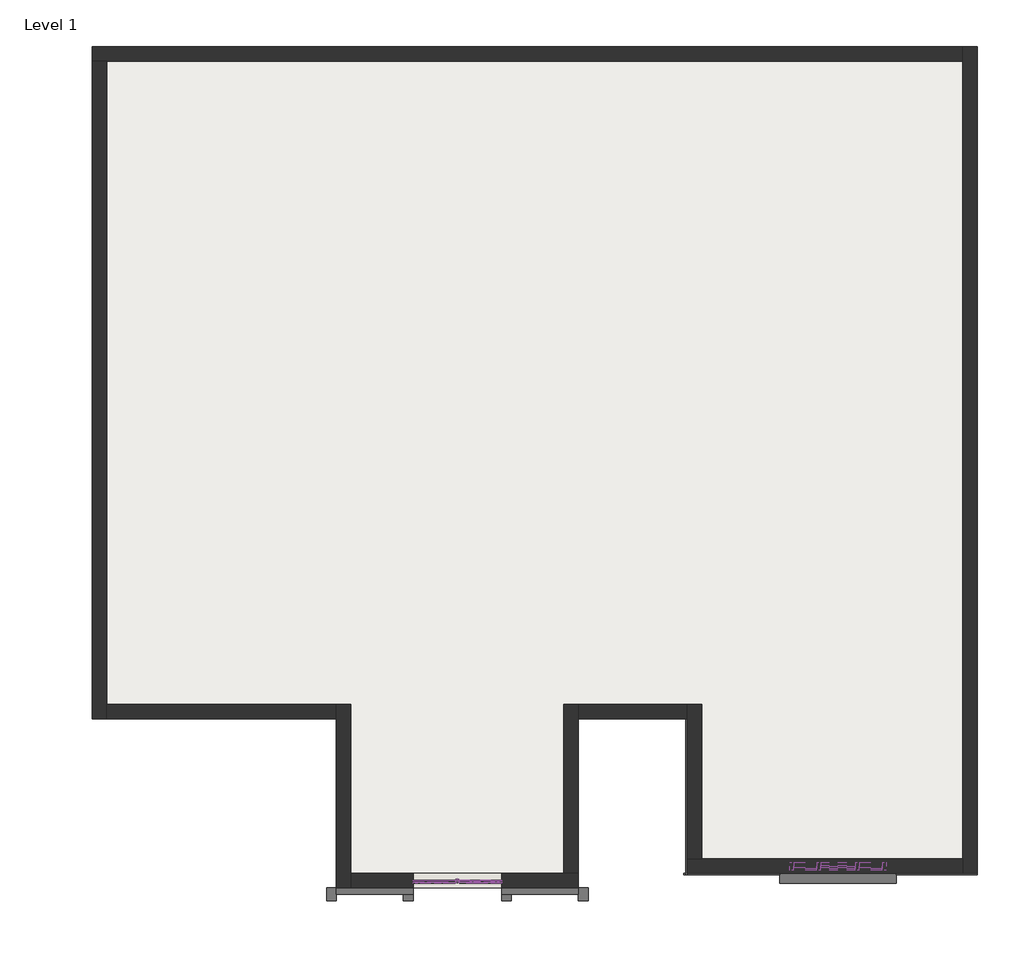
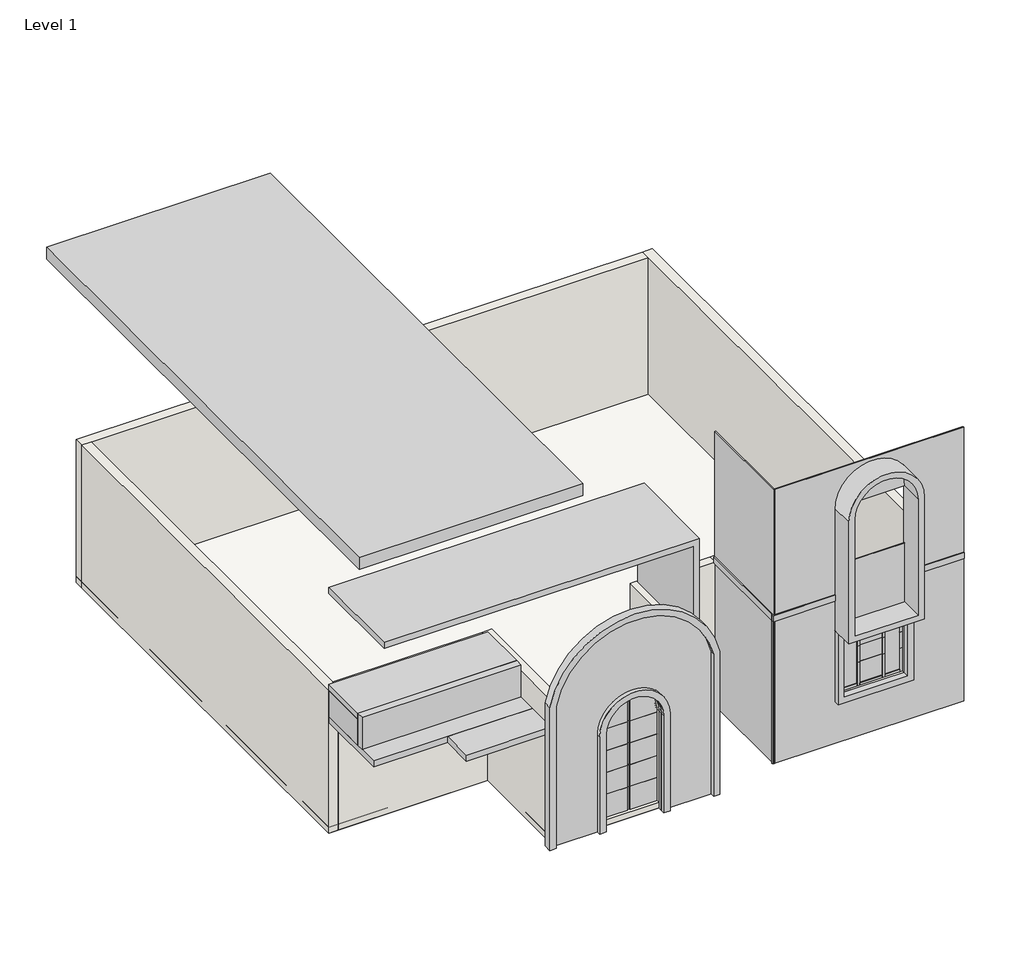
# One storey: 52 members, 17 plates, 10 walls, 1 proxy, 1 slab.
"""IFC4 building model written with IfcOpenShell, lengths in millimetres."""

from ifc_helpers import new_model, si_unit, frame, origin, origin_with_axes, place, context, project, spatial, polyline, circle_curve, outline, extrude, faceted_brep, transform, mapped, element, save
from ifc_brep_helpers import plane_surface, revolved_surface, advanced_brep
from components import generic_models_1_generic_models_1_ec26760c, member_08c7225e, member_28930b13, member_e49bab3c, member_1c8f807b, member_b3cb6624, member_4e015be9, member_3b441234, member_02ee8d56, member_e1a7572e, member_43115751, member_bd529d22, member_a55882dd, member_6e035839, member_ea2f4e14, member_6b6d42fb, member_11e54509, member_471b44ca, member_90750a43, member_576e3203, member_843225dc, member_a980948f, member_7fd687a9, member_94122dd8, member_cc20b924, system_panel_glazed_54165e4b, system_panel_glazed_81b96659, system_panel_glazed_ec3758d8, system_panel_glazed_692768b6, system_panel_glazed_4eb050cd, system_panel_glazed_dbe48e5a, system_panel_glazed_09ca6336, system_panel_glazed_22d47ebb, system_panel_glazed_ec18a58b, system_panel_glazed_47dd2052

model = new_model("IFC4")

# Units and contexts
model_context = context("Model", 3, world=origin())
ifc_project = project(units=[si_unit("LENGTHUNIT", "METRE", prefix="MILLI")], contexts=[model_context])

# Site, building, storey
site = spatial("IfcSite", under=ifc_project)
building = spatial("IfcBuilding", under=site)
storey = spatial("IfcBuildingStorey", under=building, Name="Level 1", Elevation=0.0)

# Proxy
placement = place(None, origin())
generic_models_1_generic_models_1_shape = generic_models_1_generic_models_1_ec26760c(model_context)
element("IfcBuildingElementProxy", 1, Name="Generic Models 1 : Generic Models 1", ObjectType="Generic Models 1 : Generic Models 1", at=placement, inside=storey, context=model_context, shape_type="MappedRepresentation", body=[
    mapped(generic_models_1_generic_models_1_shape, transform((0.0, 0.0, 0.0), x_axis=(1.0, 0.0, 0.0), y_axis=(0.0, 1.0, 0.0), z_axis=(0.0, 0.0, 1.0))),
])

# Members
member_shape = member_08c7225e(model_context)
element("IfcMember", 2, ObjectType="Circular Mullion : 2.5\" Circular", at=placement, inside=storey, context=model_context, shape_type="MappedRepresentation", body=[
    mapped(member_shape, transform((-633.8864268, -1847.4234736, 745.0666667), x_axis=(-1.0, 0.0, 0.0), y_axis=(0.0, 1.0, 0.0), z_axis=(0.0, 0.0, -1.0))),
])
element("IfcMember", 3, ObjectType="Circular Mullion : 2.5\" Circular", at=placement, inside=storey, context=model_context, shape_type="MappedRepresentation", body=[
    mapped(member_shape, transform((-633.8864268, -1847.4234736, 1303.8666667), x_axis=(-1.0, 0.0, 0.0), y_axis=(0.0, 1.0, 0.0), z_axis=(0.0, 0.0, -1.0))),
])
element("IfcMember", 4, ObjectType="Circular Mullion : 2.5\" Circular", at=placement, inside=storey, context=model_context, shape_type="MappedRepresentation", body=[
    mapped(member_shape, transform((-633.8864268, -1847.4234736, 1862.6666667), x_axis=(-1.0, 0.0, 0.0), y_axis=(0.0, 1.0, 0.0), z_axis=(0.0, 0.0, -1.0))),
])
member_2_shape = member_28930b13(model_context)
element("IfcMember", 5, ObjectType="Circular Mullion : 2.5\" Circular", at=placement, inside=storey, context=model_context, shape_type="MappedRepresentation", body=[
    mapped(member_2_shape, transform((-633.8864268, -1847.4234736, 2421.4666667), x_axis=(-1.0, 0.0, 0.0), y_axis=(0.0, 1.0, 0.0), z_axis=(0.0, 0.0, -1.0))),
])
member_3_shape = member_e49bab3c(model_context)
element("IfcMember", 6, ObjectType="Circular Mullion : 2.5\" Circular", at=placement, inside=storey, context=model_context, shape_type="MappedRepresentation", body=[
    mapped(member_3_shape, transform((-633.8864268, -1847.4234736, 3048.0), x_axis=(-1.0, 0.0, 0.0), y_axis=(0.0, 1.0, 0.0), z_axis=(0.0, 0.0, -1.0))),
])
member_4_shape = member_1c8f807b(model_context)
element("IfcMember", 7, ObjectType="Circular Mullion : 2.5\" Circular", at=placement, inside=storey, context=model_context, shape_type="MappedRepresentation", body=[
    mapped(member_4_shape, transform((-633.8864268, -1847.4234736, 152.4), x_axis=(-1.0, 0.0, 0.0), y_axis=(0.0, 1.0, 0.0), z_axis=(0.0, 0.0, -1.0))),
])
member_5_shape = member_b3cb6624(model_context)
element("IfcMember", 8, ObjectType="Circular Mullion : 2.5\" Circular 2", at=placement, inside=storey, context=model_context, shape_type="MappedRepresentation", body=[
    mapped(member_5_shape, transform((-1052.9864268, -1847.4234736, 3048.0), x_axis=(0.0, 0.0, 1.0), y_axis=(0.0, 1.0, 0.0), z_axis=(-1.0, 0.0, 0.0))),
])
element("IfcMember", 9, ObjectType="Circular Mullion : 2.5\" Circular 2", at=placement, inside=storey, context=model_context, shape_type="MappedRepresentation", body=[
    mapped(member_5_shape, transform((-602.1364268, -1847.4234736, 3048.0), x_axis=(0.0, 0.0, 1.0), y_axis=(0.0, 1.0, 0.0), z_axis=(-1.0, 0.0, 0.0))),
])
member_6_shape = member_4e015be9(model_context)
element("IfcMember", 10, ObjectType="Circular Mullion : 2.5\" Circular 2", at=placement, inside=storey, context=model_context, shape_type="MappedRepresentation", body=[
    mapped(member_6_shape, transform((-1325.1474268, -1847.4234736, 1862.6666667), x_axis=(0.0, 0.0, 1.0), y_axis=(0.0, 1.0, 0.0), z_axis=(-1.0, 0.0, 0.0))),
])
element("IfcMember", 11, ObjectType="Circular Mullion : 2.5\" Circular 2", at=placement, inside=storey, context=model_context, shape_type="MappedRepresentation", body=[
    mapped(member_6_shape, transform((-602.1364268, -1847.4234736, 1862.6666667), x_axis=(0.0, 0.0, 1.0), y_axis=(0.0, 1.0, 0.0), z_axis=(-1.0, 0.0, 0.0))),
])
element("IfcMember", 12, ObjectType="Circular Mullion : 2.5\" Circular 2", at=placement, inside=storey, context=model_context, shape_type="MappedRepresentation", body=[
    mapped(member_6_shape, transform((-1325.1474268, -1847.4234736, 1303.8666667), x_axis=(0.0, 0.0, 1.0), y_axis=(0.0, 1.0, 0.0), z_axis=(-1.0, 0.0, 0.0))),
])
element("IfcMember", 13, ObjectType="Circular Mullion : 2.5\" Circular 2", at=placement, inside=storey, context=model_context, shape_type="MappedRepresentation", body=[
    mapped(member_6_shape, transform((-602.1364268, -1847.4234736, 1303.8666667), x_axis=(0.0, 0.0, 1.0), y_axis=(0.0, 1.0, 0.0), z_axis=(-1.0, 0.0, 0.0))),
])
element("IfcMember", 14, ObjectType="Circular Mullion : 2.5\" Circular 2", at=placement, inside=storey, context=model_context, shape_type="MappedRepresentation", body=[
    mapped(member_6_shape, transform((-1325.1474268, -1847.4234736, 745.0666667), x_axis=(0.0, 0.0, 1.0), y_axis=(0.0, 1.0, 0.0), z_axis=(-1.0, 0.0, 0.0))),
])
element("IfcMember", 15, ObjectType="Circular Mullion : 2.5\" Circular 2", at=placement, inside=storey, context=model_context, shape_type="MappedRepresentation", body=[
    mapped(member_6_shape, transform((-602.1364268, -1847.4234736, 745.0666667), x_axis=(0.0, 0.0, 1.0), y_axis=(0.0, 1.0, 0.0), z_axis=(-1.0, 0.0, 0.0))),
])
element("IfcMember", 16, ObjectType="Circular Mullion : 2.5\" Circular 2", at=placement, inside=storey, context=model_context, shape_type="MappedRepresentation", body=[
    mapped(member_6_shape, transform((-1325.1474268, -1847.4234736, 2421.4666667), x_axis=(0.0, 0.0, 1.0), y_axis=(0.0, 1.0, 0.0), z_axis=(-1.0, 0.0, 0.0))),
])
member_7_shape = member_3b441234(model_context)
element("IfcMember", 17, ObjectType="Circular Mullion : 2.5\" Circular 2", at=placement, inside=storey, context=model_context, shape_type="MappedRepresentation", body=[
    mapped(member_7_shape, transform((64.6135732, -1847.4234736, 2489.2), x_axis=(1.0, 0.0, 0.0), y_axis=(0.0, 1.0, 0.0), z_axis=(0.0, 0.0, 1.0))),
])
member_8_shape = member_02ee8d56(model_context)
element("IfcMember", 18, ObjectType="Circular Mullion : 2.5\" Circular 2", at=placement, inside=storey, context=model_context, shape_type="MappedRepresentation", body=[
    mapped(member_8_shape, transform((-1332.3864268, -1847.4234736, 152.4), x_axis=(-1.0, 0.0, 0.0), y_axis=(0.0, 1.0, 0.0), z_axis=(0.0, 0.0, -1.0))),
])
member_9_shape = member_e1a7572e(model_context)
element("IfcMember", 19, ObjectType="Circular Mullion : 2.5\" Circular 2", at=placement, inside=storey, context=model_context, shape_type="MappedRepresentation", body=[
    mapped(member_9_shape, transform((57.3745732, -1847.4234736, 152.4), x_axis=(0.0, 0.0, -1.0), y_axis=(0.0, 1.0, 0.0), z_axis=(1.0, 0.0, 0.0))),
])
element("IfcMember", 20, ObjectType="Circular Mullion : 2.5\" Circular 2", at=placement, inside=storey, context=model_context, shape_type="MappedRepresentation", body=[
    mapped(member_9_shape, transform((-665.6364268, -1847.4234736, 152.4), x_axis=(0.0, 0.0, -1.0), y_axis=(0.0, 1.0, 0.0), z_axis=(1.0, 0.0, 0.0))),
])
member_10_shape = member_43115751(model_context)
element("IfcMember", 21, ObjectType="Circular Mullion : 2.5\" Circular 2", at=placement, inside=storey, context=model_context, shape_type="MappedRepresentation", body=[
    mapped(member_10_shape, transform((-1332.3864268, -1847.4234736, 2489.2), x_axis=(-1.0, 0.0, 0.0), y_axis=(0.0, 1.0, 0.0), z_axis=(0.0, 0.0, -1.0))),
])
element("IfcMember", 22, ObjectType="Circular Mullion : 2.5\" Circular 2", at=placement, inside=storey, context=model_context, shape_type="MappedRepresentation", body=[
    mapped(member_7_shape, transform((-1332.3864268, -1847.4234736, 2421.4666667), x_axis=(-1.0, 0.0, 0.0), y_axis=(0.0, 1.0, 0.0), z_axis=(0.0, 0.0, -1.0))),
])
member_11_shape = member_bd529d22(model_context)
element("IfcMember", 23, ObjectType="Circular Mullion : 2.5\" Circular 2", at=placement, inside=storey, context=model_context, shape_type="MappedRepresentation", body=[
    mapped(member_11_shape, transform((-1332.3864268, -1847.4234736, 1862.6666667), x_axis=(-1.0, 0.0, 0.0), y_axis=(0.0, 1.0, 0.0), z_axis=(0.0, 0.0, -1.0))),
])
element("IfcMember", 24, ObjectType="Circular Mullion : 2.5\" Circular 2", at=placement, inside=storey, context=model_context, shape_type="MappedRepresentation", body=[
    mapped(member_11_shape, transform((-1332.3864268, -1847.4234736, 1303.8666667), x_axis=(-1.0, 0.0, 0.0), y_axis=(0.0, 1.0, 0.0), z_axis=(0.0, 0.0, -1.0))),
])
element("IfcMember", 25, ObjectType="Circular Mullion : 2.5\" Circular 2", at=placement, inside=storey, context=model_context, shape_type="MappedRepresentation", body=[
    mapped(member_11_shape, transform((-1332.3864268, -1847.4234736, 745.0666667), x_axis=(-1.0, 0.0, 0.0), y_axis=(0.0, 1.0, 0.0), z_axis=(0.0, 0.0, -1.0))),
])
element("IfcMember", 26, ObjectType="Circular Mullion : 2.5\" Circular 2", at=placement, inside=storey, context=model_context, shape_type="MappedRepresentation", body=[
    mapped(member_11_shape, transform((64.6135732, -1847.4234736, 2421.4666667), x_axis=(1.0, 0.0, 0.0), y_axis=(0.0, 1.0, 0.0), z_axis=(0.0, 0.0, 1.0))),
])
element("IfcMember", 27, ObjectType="Circular Mullion : 2.5\" Circular 2", at=placement, inside=storey, context=model_context, shape_type="MappedRepresentation", body=[
    mapped(member_11_shape, transform((64.6135732, -1847.4234736, 1862.6666667), x_axis=(1.0, 0.0, 0.0), y_axis=(0.0, 1.0, 0.0), z_axis=(0.0, 0.0, 1.0))),
])
element("IfcMember", 28, ObjectType="Circular Mullion : 2.5\" Circular 2", at=placement, inside=storey, context=model_context, shape_type="MappedRepresentation", body=[
    mapped(member_11_shape, transform((64.6135732, -1847.4234736, 1303.8666667), x_axis=(1.0, 0.0, 0.0), y_axis=(0.0, 1.0, 0.0), z_axis=(0.0, 0.0, 1.0))),
])
element("IfcMember", 29, ObjectType="Circular Mullion : 2.5\" Circular 2", at=placement, inside=storey, context=model_context, shape_type="MappedRepresentation", body=[
    mapped(member_8_shape, transform((64.6135732, -1847.4234736, 745.0666667), x_axis=(1.0, 0.0, 0.0), y_axis=(0.0, 1.0, 0.0), z_axis=(0.0, 0.0, 1.0))),
])
member_12_shape = member_a55882dd(model_context)
element("IfcMember", 30, ObjectType="Circular Mullion : 2.5\" Circular 2", at=placement, inside=storey, context=model_context, shape_type="MappedRepresentation", body=[
    mapped(member_12_shape, transform((-633.8864268, -1847.4234736, 3187.7), x_axis=(0.0, 0.0, 1.0), y_axis=(0.0, 1.0, 0.0), z_axis=(-1.0, 0.0, 0.0))),
])
member_13_shape = member_6e035839(model_context)
element("IfcMember", 31, ObjectType="Circular Mullion : 2.5\" Circular 2", at=placement, inside=storey, context=model_context, shape_type="MappedRepresentation", body=[
    mapped(member_13_shape, transform((-214.7864268, -1847.4234736, 3048.0), x_axis=(0.5999999999999911, 0.0, 0.8000000000000067), y_axis=(0.0, 1.0, 0.0), z_axis=(-0.8000000000000067, 0.0, 0.5999999999999911))),
])
member_14_shape = member_ea2f4e14(model_context)
element("IfcMember", 32, ObjectType="Circular Mullion : 2.5\" Circular 2", at=placement, inside=storey, context=model_context, shape_type="MappedRepresentation", body=[
    mapped(member_14_shape, transform((-1052.9864268, -1847.4234736, 3048.0), x_axis=(-0.5999999999999878, 0.0, 0.8000000000000093), y_axis=(0.0, 1.0, 0.0), z_axis=(-0.8000000000000091, 0.0, -0.5999999999999877))),
])
member_15_shape = member_6b6d42fb(model_context)
element("IfcMember", 33, ObjectType="Rectangular Mullion : 1\" Square", at=placement, inside=storey, context=model_context, shape_type="MappedRepresentation", body=[
    mapped(member_15_shape, transform((-602.1364268, -1847.4234736, 2421.4666667), x_axis=(0.0, 0.0, 1.0), y_axis=(0.0, 1.0, 0.0), z_axis=(-1.0, 0.0, 0.0))),
])
member_16_shape = member_11e54509(model_context)
element("IfcMember", 34, ObjectType="Rectangular Mullion : 1\" Square", at=placement, inside=storey, context=model_context, shape_type="MappedRepresentation", body=[
    mapped(member_16_shape, transform((5087.4635732, -1618.8234736, 2235.2), x_axis=(0.0, 0.0, 1.0), y_axis=(0.0, 1.0, 0.0), z_axis=(-1.0, 0.0, 0.0))),
])
element("IfcMember", 35, ObjectType="Rectangular Mullion : 1\" Square", at=placement, inside=storey, context=model_context, shape_type="MappedRepresentation", body=[
    mapped(member_16_shape, transform((5087.4635732, -1618.8234736, 1820.3333333), x_axis=(0.0, 0.0, 1.0), y_axis=(0.0, 1.0, 0.0), z_axis=(-1.0, 0.0, 0.0))),
])
member_17_shape = member_471b44ca(model_context)
element("IfcMember", 36, ObjectType="Rectangular Mullion : 2.5\" x 5\" rectangular", at=placement, inside=storey, context=model_context, shape_type="MappedRepresentation", body=[
    mapped(member_17_shape, transform((5055.7135732, -1618.8234736, 1820.3333333), x_axis=(-1.0, 0.0, 0.0), y_axis=(0.0, 1.0, 0.0), z_axis=(0.0, 0.0, -1.0))),
])
element("IfcMember", 37, ObjectType="Rectangular Mullion : 2.5\" x 5\" rectangular", at=placement, inside=storey, context=model_context, shape_type="MappedRepresentation", body=[
    mapped(member_17_shape, transform((5665.3135732, -1618.8234736, 1820.3333333), x_axis=(-1.0, 0.0, 0.0), y_axis=(0.0, 1.0, 0.0), z_axis=(0.0, 0.0, -1.0))),
])
member_18_shape = member_90750a43(model_context)
element("IfcMember", 38, ObjectType="Rectangular Mullion : 2.5\" x 5\" rectangular", at=placement, inside=storey, context=model_context, shape_type="MappedRepresentation", body=[
    mapped(member_18_shape, transform((5055.7135732, -1618.8234736, 2235.2), x_axis=(-1.0, 0.0, 0.0), y_axis=(0.0, 1.0, 0.0), z_axis=(0.0, 0.0, -1.0))),
])
element("IfcMember", 39, ObjectType="Rectangular Mullion : 2.5\" x 5\" rectangular", at=placement, inside=storey, context=model_context, shape_type="MappedRepresentation", body=[
    mapped(member_18_shape, transform((5665.3135732, -1618.8234736, 2235.2), x_axis=(-1.0, 0.0, 0.0), y_axis=(0.0, 1.0, 0.0), z_axis=(0.0, 0.0, -1.0))),
])
member_19_shape = member_576e3203(model_context)
element("IfcMember", 40, ObjectType="Rectangular Mullion : 2.5\" x 5\" rectangular", at=placement, inside=storey, context=model_context, shape_type="MappedRepresentation", body=[
    mapped(member_19_shape, transform((5055.7135732, -1618.8234736, 1219.2), x_axis=(-1.0, 0.0, 0.0), y_axis=(0.0, 1.0, 0.0), z_axis=(0.0, 0.0, -1.0))),
])
element("IfcMember", 41, ObjectType="Rectangular Mullion : 2.5\" x 5\" rectangular", at=placement, inside=storey, context=model_context, shape_type="MappedRepresentation", body=[
    mapped(member_19_shape, transform((5665.3135732, -1618.8234736, 1219.2), x_axis=(-1.0, 0.0, 0.0), y_axis=(0.0, 1.0, 0.0), z_axis=(0.0, 0.0, -1.0))),
])
member_20_shape = member_843225dc(model_context)
element("IfcMember", 42, ObjectType="Rectangular Mullion : 2.5\" x 5\" rectangular", at=placement, inside=storey, context=model_context, shape_type="MappedRepresentation", body=[
    mapped(member_20_shape, transform((4662.0135732, -1618.8234736, 2743.2), x_axis=(0.0, 0.0, 1.0), y_axis=(0.0, 1.0, 0.0), z_axis=(-1.0, 0.0, 0.0))),
])
element("IfcMember", 43, ObjectType="Rectangular Mullion : 2.5\" x 5\" rectangular", at=placement, inside=storey, context=model_context, shape_type="MappedRepresentation", body=[
    mapped(member_20_shape, transform((5697.0635732, -1618.8234736, 2743.2), x_axis=(0.0, 0.0, 1.0), y_axis=(0.0, 1.0, 0.0), z_axis=(-1.0, 0.0, 0.0))),
])
element("IfcMember", 44, ObjectType="Rectangular Mullion : 2.5\" x 5\" rectangular", at=placement, inside=storey, context=model_context, shape_type="MappedRepresentation", body=[
    mapped(member_20_shape, transform((6059.0135732, -1618.8234736, 1219.2), x_axis=(0.0, 0.0, -1.0), y_axis=(0.0, 1.0, 0.0), z_axis=(1.0, 0.0, 0.0))),
])
element("IfcMember", 45, ObjectType="Rectangular Mullion : 2.5\" x 5\" rectangular", at=placement, inside=storey, context=model_context, shape_type="MappedRepresentation", body=[
    mapped(member_20_shape, transform((5023.9635732, -1618.8234736, 1219.2), x_axis=(0.0, 0.0, -1.0), y_axis=(0.0, 1.0, 0.0), z_axis=(1.0, 0.0, 0.0))),
])
member_21_shape = member_a980948f(model_context)
element("IfcMember", 46, ObjectType="Rectangular Mullion : 2.5\" x 5\" rectangular", at=placement, inside=storey, context=model_context, shape_type="MappedRepresentation", body=[
    mapped(member_21_shape, transform((5633.5635732, -1618.8234736, 1219.2), x_axis=(0.0, 0.0, -1.0), y_axis=(0.0, 1.0, 0.0), z_axis=(1.0, 0.0, 0.0))),
])
element("IfcMember", 47, ObjectType="Rectangular Mullion : 2.5\" x 5\" rectangular", at=placement, inside=storey, context=model_context, shape_type="MappedRepresentation", body=[
    mapped(member_21_shape, transform((5087.4635732, -1618.8234736, 2743.2), x_axis=(0.0, 0.0, 1.0), y_axis=(0.0, 1.0, 0.0), z_axis=(-1.0, 0.0, 0.0))),
])
member_22_shape = member_7fd687a9(model_context)
element("IfcMember", 48, ObjectType="Rectangular Mullion : 2.5\" x 5\" rectangular", at=placement, inside=storey, context=model_context, shape_type="MappedRepresentation", body=[
    mapped(member_22_shape, transform((6122.5135732, -1618.8234736, 2743.2), x_axis=(1.0, 0.0, 0.0), y_axis=(0.0, 1.0, 0.0), z_axis=(0.0, 0.0, 1.0))),
])
member_23_shape = member_94122dd8(model_context)
element("IfcMember", 49, ObjectType="Rectangular Mullion : 2.5\" x 5\" rectangular", at=placement, inside=storey, context=model_context, shape_type="MappedRepresentation", body=[
    mapped(member_23_shape, transform((4598.5135732, -1618.8234736, 1219.2), x_axis=(-1.0, 0.0, 0.0), y_axis=(0.0, 1.0, 0.0), z_axis=(0.0, 0.0, -1.0))),
])
element("IfcMember", 50, ObjectType="Rectangular Mullion : 2.5\" x 5\" rectangular", at=placement, inside=storey, context=model_context, shape_type="MappedRepresentation", body=[
    mapped(member_22_shape, transform((4598.5135732, -1618.8234736, 2235.2), x_axis=(-1.0, 0.0, 0.0), y_axis=(0.0, 1.0, 0.0), z_axis=(0.0, 0.0, -1.0))),
])
member_24_shape = member_cc20b924(model_context)
element("IfcMember", 51, ObjectType="Rectangular Mullion : 2.5\" x 5\" rectangular", at=placement, inside=storey, context=model_context, shape_type="MappedRepresentation", body=[
    mapped(member_24_shape, transform((4598.5135732, -1618.8234736, 1820.3333333), x_axis=(-1.0, 0.0, 0.0), y_axis=(0.0, 1.0, 0.0), z_axis=(0.0, 0.0, -1.0))),
])
element("IfcMember", 52, ObjectType="Rectangular Mullion : 2.5\" x 5\" rectangular", at=placement, inside=storey, context=model_context, shape_type="MappedRepresentation", body=[
    mapped(member_24_shape, transform((6122.5135732, -1618.8234736, 2235.2), x_axis=(1.0, 0.0, 0.0), y_axis=(0.0, 1.0, 0.0), z_axis=(0.0, 0.0, 1.0))),
])
element("IfcMember", 53, ObjectType="Rectangular Mullion : 2.5\" x 5\" rectangular", at=placement, inside=storey, context=model_context, shape_type="MappedRepresentation", body=[
    mapped(member_23_shape, transform((6122.5135732, -1618.8234736, 1820.3333333), x_axis=(1.0, 0.0, 0.0), y_axis=(0.0, 1.0, 0.0), z_axis=(0.0, 0.0, 1.0))),
])

# Plates
system_panel_glazed_shape = system_panel_glazed_54165e4b(model_context)
element("IfcPlate", 54, ObjectType="System Panel : Glazed", at=placement, inside=storey, context=model_context, shape_type="MappedRepresentation", body=[
    mapped(system_panel_glazed_shape, transform((-268.7614268, -1847.4234736, 152.4), x_axis=(-1.0, 0.0, 0.0), y_axis=(0.0, -1.0, 0.0), z_axis=(0.0, 0.0, 1.0))),
])
element("IfcPlate", 55, ObjectType="System Panel : Glazed", at=placement, inside=storey, context=model_context, shape_type="MappedRepresentation", body=[
    mapped(system_panel_glazed_shape, transform((-999.0114268, -1847.4234736, 152.4), x_axis=(-1.0, 0.0, 0.0), y_axis=(0.0, -1.0, 0.0), z_axis=(0.0, 0.0, 1.0))),
])
system_panel_glazed_2_shape = system_panel_glazed_81b96659(model_context)
element("IfcPlate", 56, ObjectType="System Panel : Glazed", at=placement, inside=storey, context=model_context, shape_type="MappedRepresentation", body=[
    mapped(system_panel_glazed_2_shape, transform((-408.4614268, -1847.4234736, 3048.0), x_axis=(-1.0, 0.0, 0.0), y_axis=(0.0, -1.0, 0.0), z_axis=(0.0, 0.0, 1.0))),
])
system_panel_glazed_3_shape = system_panel_glazed_ec3758d8(model_context)
element("IfcPlate", 57, ObjectType="System Panel : Glazed", at=placement, inside=storey, context=model_context, shape_type="MappedRepresentation", body=[
    mapped(system_panel_glazed_3_shape, transform((-859.3114268, -1847.4234736, 3048.0), x_axis=(-1.0, 0.0, 0.0), y_axis=(0.0, -1.0, 0.0), z_axis=(0.0, 0.0, 1.0))),
])
system_panel_glazed_4_shape = system_panel_glazed_692768b6(model_context)
element("IfcPlate", 58, ObjectType="System Panel : Glazed", at=placement, inside=storey, context=model_context, shape_type="MappedRepresentation", body=[
    mapped(system_panel_glazed_4_shape, transform((-268.7614268, -1847.4234736, 1862.6666667), x_axis=(-1.0, 0.0, 0.0), y_axis=(0.0, -1.0, 0.0), z_axis=(0.0, 0.0, 1.0))),
])
element("IfcPlate", 59, ObjectType="System Panel : Glazed", at=placement, inside=storey, context=model_context, shape_type="MappedRepresentation", body=[
    mapped(system_panel_glazed_4_shape, transform((-999.0114268, -1847.4234736, 1862.6666667), x_axis=(-1.0, 0.0, 0.0), y_axis=(0.0, -1.0, 0.0), z_axis=(0.0, 0.0, 1.0))),
])
element("IfcPlate", 60, ObjectType="System Panel : Glazed", at=placement, inside=storey, context=model_context, shape_type="MappedRepresentation", body=[
    mapped(system_panel_glazed_4_shape, transform((-268.7614268, -1847.4234736, 1303.8666667), x_axis=(-1.0, 0.0, 0.0), y_axis=(0.0, -1.0, 0.0), z_axis=(0.0, 0.0, 1.0))),
])
element("IfcPlate", 61, ObjectType="System Panel : Glazed", at=placement, inside=storey, context=model_context, shape_type="MappedRepresentation", body=[
    mapped(system_panel_glazed_4_shape, transform((-999.0114268, -1847.4234736, 1303.8666667), x_axis=(-1.0, 0.0, 0.0), y_axis=(0.0, -1.0, 0.0), z_axis=(0.0, 0.0, 1.0))),
])
element("IfcPlate", 62, ObjectType="System Panel : Glazed", at=placement, inside=storey, context=model_context, shape_type="MappedRepresentation", body=[
    mapped(system_panel_glazed_4_shape, transform((-268.7614268, -1847.4234736, 745.0666667), x_axis=(-1.0, 0.0, 0.0), y_axis=(0.0, -1.0, 0.0), z_axis=(0.0, 0.0, 1.0))),
])
element("IfcPlate", 63, ObjectType="System Panel : Glazed", at=placement, inside=storey, context=model_context, shape_type="MappedRepresentation", body=[
    mapped(system_panel_glazed_4_shape, transform((-999.0114268, -1847.4234736, 745.0666667), x_axis=(-1.0, 0.0, 0.0), y_axis=(0.0, -1.0, 0.0), z_axis=(0.0, 0.0, 1.0))),
])
system_panel_glazed_5_shape = system_panel_glazed_4eb050cd(model_context)
element("IfcPlate", 64, ObjectType="System Panel : Glazed", at=placement, inside=storey, context=model_context, shape_type="MappedRepresentation", body=[
    mapped(system_panel_glazed_5_shape, transform((-268.7614268, -1847.4234736, 2421.4666667), x_axis=(-1.0, 0.0, 0.0), y_axis=(0.0, -1.0, 0.0), z_axis=(0.0, 0.0, 1.0))),
])
system_panel_glazed_6_shape = system_panel_glazed_dbe48e5a(model_context)
element("IfcPlate", 65, ObjectType="System Panel : Glazed", at=placement, inside=storey, context=model_context, shape_type="MappedRepresentation", body=[
    mapped(system_panel_glazed_6_shape, transform((-999.0114268, -1847.4234736, 2421.4666667), x_axis=(-1.0, 0.0, 0.0), y_axis=(0.0, -1.0, 0.0), z_axis=(0.0, 0.0, 1.0))),
])
system_panel_glazed_7_shape = system_panel_glazed_09ca6336(model_context)
element("IfcPlate", 66, ObjectType="System Panel : Glazed", at=placement, inside=storey, context=model_context, shape_type="MappedRepresentation", body=[
    mapped(system_panel_glazed_7_shape, transform((5360.5135732, -1618.8234736, 1820.3333333), x_axis=(-1.0, 0.0, 0.0), y_axis=(0.0, -1.0, 0.0), z_axis=(0.0, 0.0, 1.0))),
])
system_panel_glazed_8_shape = system_panel_glazed_22d47ebb(model_context)
element("IfcPlate", 67, ObjectType="System Panel : Glazed", at=placement, inside=storey, context=model_context, shape_type="MappedRepresentation", body=[
    mapped(system_panel_glazed_8_shape, transform((5878.0385732, -1618.8234736, 1282.7), x_axis=(-1.0, 0.0, 0.0), y_axis=(0.0, -1.0, 0.0), z_axis=(0.0, 0.0, 1.0))),
])
element("IfcPlate", 68, ObjectType="System Panel : Glazed", at=placement, inside=storey, context=model_context, shape_type="MappedRepresentation", body=[
    mapped(system_panel_glazed_8_shape, transform((4842.9885732, -1618.8234736, 1282.7), x_axis=(-1.0, 0.0, 0.0), y_axis=(0.0, -1.0, 0.0), z_axis=(0.0, 0.0, 1.0))),
])
system_panel_glazed_9_shape = system_panel_glazed_ec18a58b(model_context)
element("IfcPlate", 69, ObjectType="System Panel : Glazed", at=placement, inside=storey, context=model_context, shape_type="MappedRepresentation", body=[
    mapped(system_panel_glazed_9_shape, transform((5360.5135732, -1618.8234736, 1282.7), x_axis=(-1.0, 0.0, 0.0), y_axis=(0.0, -1.0, 0.0), z_axis=(0.0, 0.0, 1.0))),
])
system_panel_glazed_10_shape = system_panel_glazed_47dd2052(model_context)
element("IfcPlate", 70, ObjectType="System Panel : Glazed", at=placement, inside=storey, context=model_context, shape_type="MappedRepresentation", body=[
    mapped(system_panel_glazed_10_shape, transform((5360.5135732, -1618.8234736, 2235.2), x_axis=(-1.0, 0.0, 0.0), y_axis=(0.0, -1.0, 0.0), z_axis=(0.0, 0.0, 1.0))),
])

# Slab
element("IfcSlab", 71, ObjectType="6\" GF", at=placement, inside=storey, context=model_context, shape_type="SweptSolid", body=[
    extrude(outline(polyline([(-6386.9864268, 11297.0765264), (7557.6135732, 11297.0765264), (7557.6135732, -1733.1234736), (2985.6135732, -1733.1234736), (2985.6135732, 705.2765264), (1271.1135732, 705.2765264), (1271.1135732, -1961.7234736), (-2538.8864268, -1961.7234736), (-2538.8864268, 705.2765264), (-6386.9864268, 705.2765264), (-6386.9864268, 11297.0765264)])), origin_with_axes(), (0.0, 0.0, 1.0), 152.4),
])

# Walls
element("IfcWall", 72, ObjectType="9\" wall", at=placement, inside=storey, context=model_context, shape_type="Brep", body=[
    faceted_brep([(-6386.9864268, 11068.4765264, 0.0), (-6158.3864268, 11068.4765264, 0.0), (7329.0135732, 11068.4765264, 0.0), (7329.0135732, 11068.4765264, 3657.6), (-6158.3864268, 11068.4765264, 3657.6), (-6386.9864268, 11068.4765264, 3657.6), (-6386.9864268, 11297.0765264, 0.0), (-6386.9864268, 11297.0765264, 3657.6), (7329.0135732, 11297.0765264, 3657.6), (7329.0135732, 11297.0765264, 0.0)], [[[0, 1, 2, 3, 4, 5]], [[6, 7, 8, 9]], [[2, 1, 0, 6, 9]], [[0, 5, 7, 6]], [[3, 2, 9, 8]], [[5, 4, 3, 8, 7]]]),
])
element("IfcWall", 73, ObjectType="9\" wall", at=placement, inside=storey, context=model_context, shape_type="Brep", body=[
    faceted_brep([(-6158.3864268, 705.2765264, 0.0), (-6158.3864268, 933.8765264, 0.0), (-6158.3864268, 11068.4765264, 0.0), (-6158.3864268, 11068.4765264, 3657.6), (-6158.3864268, 933.8765264, 3657.6), (-6158.3864268, 705.2765264, 3657.6), (-6386.9864268, 705.2765264, 0.0), (-6386.9864268, 705.2765264, 3657.6), (-6386.9864268, 11068.4765264, 3657.6), (-6386.9864268, 11068.4765264, 0.0)], [[[0, 1, 2, 3, 4, 5]], [[6, 7, 8, 9]], [[2, 1, 0, 6, 9]], [[0, 5, 7, 6]], [[3, 2, 9, 8]], [[5, 4, 3, 8, 7]]]),
])
element("IfcWall", 74, ObjectType="9\" wall", at=placement, inside=storey, context=model_context, shape_type="Brep", body=[
    faceted_brep([(7329.0135732, 11297.0765264, 0.0), (7329.0135732, 11068.4765264, 0.0), (7329.0135732, -1504.5234736, 0.0), (7329.0135732, -1733.1234736, 0.0), (7329.0135732, -1733.1234736, 3657.6), (7329.0135732, -1504.5234736, 3657.6), (7329.0135732, 11068.4765264, 3657.6), (7329.0135732, 11297.0765264, 3657.6), (7557.6135732, 11297.0765264, 0.0), (7557.6135732, 11297.0765264, 3657.6), (7557.6135732, -1733.1234736, 3657.6), (7557.6135732, -1733.1234736, 0.0)], [[[0, 1, 2, 3, 4, 5, 6, 7]], [[8, 9, 10, 11]], [[3, 2, 1, 0, 8, 11]], [[0, 7, 9, 8]], [[4, 3, 11, 10]], [[7, 6, 5, 4, 10, 9]]]),
])
element("IfcWall", 75, ObjectType="9\" wall", at=placement, inside=storey, context=model_context, shape_type="Brep", body=[
    faceted_brep([(-2538.8864268, 933.8765264, 0.0), (-2538.8864268, 705.2765264, 0.0), (-2538.8864268, -1961.7234736, 0.0), (-2538.8864268, -1961.7234736, 3657.6), (-2538.8864268, 705.2765264, 3657.6), (-2538.8864268, 933.8765264, 3657.6), (-2310.2864268, 933.8765264, 0.0), (-2310.2864268, 933.8765264, 3657.6), (-2310.2864268, -1733.1234736, 3657.6), (-2310.2864268, -1961.7234736, 3657.6), (-2310.2864268, -1961.7234736, 0.0), (-2310.2864268, -1733.1234736, 0.0)], [[[0, 1, 2, 3, 4, 5]], [[6, 7, 8, 9, 10, 11]], [[2, 1, 0, 6, 11, 10]], [[3, 2, 10, 9]], [[0, 5, 7, 6]], [[5, 4, 3, 9, 8, 7]]]),
])
element("IfcWall", 76, ObjectType="9\" wall", at=placement, inside=storey, context=model_context, shape_type="AdvancedBrep", body=[
    advanced_brep(
    [(-2310.2864268, -1961.7234736, 0.0), (1271.1135732, -1961.7234736, 0.0), (1271.1135732, -1961.7234736, 3657.6), (-2310.2864268, -1961.7234736, 3657.6), (64.6135732, -1961.7234736, 2489.2), (64.6135732, -1961.7234736, 152.4), (-1332.3864268, -1961.7234736, 152.4), (-1332.3864268, -1961.7234736, 2489.2), (1271.1135732, -1733.1234736, 0.0), (1042.5135732, -1733.1234736, 0.0), (-2310.2864268, -1733.1234736, 0.0), (-2310.2864268, -1733.1234736, 3657.6), (1042.5135732, -1733.1234736, 3657.6), (1271.1135732, -1733.1234736, 3657.6), (64.6135732, -1733.1234736, 152.4), (64.6135732, -1733.1234736, 2489.2), (-1332.3864268, -1733.1234736, 2489.2), (-1332.3864268, -1733.1234736, 152.4)],
    [
        (0, 1),
        (1, 2),
        (2, 3),
        (3, 0),
        (4, 5),
        (5, 6),
        (6, 7),
        (7, 4, circle_curve(frame((-633.8864268, -1961.7234736, 2489.2), z_axis=(0.0, 1.0, 0.0), x_axis=(1.0, 0.0, 0.0)), 698.5)),
        (8, 9),
        (9, 10),
        (10, 11),
        (11, 12),
        (12, 13),
        (13, 8),
        (14, 15),
        (15, 16, circle_curve(frame((-633.8864268, -1733.1234736, 2489.2), z_axis=(0.0, -1.0, 0.0), x_axis=(1.0, 0.0, 0.0)), 698.5)),
        (16, 17),
        (17, 14),
        (0, 10),
        (8, 1),
        (3, 11),
        (13, 2),
        (14, 5),
        (4, 15),
        (7, 16),
        (6, 17),
    ],
    [
        plane_surface(frame((-2310.2864268, -1961.7234736, 0.0), z_axis=(0.0, -1.0, 0.0), x_axis=(1.0, 0.0, 0.0))),
        plane_surface(frame((-2310.2864268, -1733.1234736, 0.0), z_axis=(0.0, 1.0, 0.0), x_axis=(-1.0, 0.0, 0.0))),
        plane_surface(frame((-2424.5864268, -1961.7234736, 0.0), z_axis=(0.0, 0.0, -1.0), x_axis=(0.0, 1.0, 0.0))),
        plane_surface(frame((-2310.2864268, 705.2765264, 0.0), z_axis=(-1.0, 0.0, 0.0), x_axis=(0.0, 1.0, 0.0))),
        plane_surface(frame((1271.1135732, -1733.1234736, 0.0), z_axis=(1.0, 0.0, 0.0), x_axis=(0.0, 1.0, 0.0))),
        plane_surface(frame((64.6135732, -2114.1234736, 152.4), z_axis=(-1.0, 0.0, 0.0), x_axis=(0.0, 1.0, 0.0))),
        revolved_surface(polyline([(64.61357320000002, -1961.7234736, 2489.2), (64.61357320000002, -1733.1234736, 2489.2)]), (-633.8864268, -1860.1234736, 2489.2), (0.0, -1.0, 0.0)),
        plane_surface(frame((-1332.3864268, -2114.1234736, 2489.2), z_axis=(1.0, 0.0, 0.0), x_axis=(0.0, 1.0, 0.0))),
        plane_surface(frame((-1332.3864268, -2114.1234736, 152.4), z_axis=(0.0, 0.0, 1.0), x_axis=(0.0, 1.0, 0.0))),
        plane_surface(frame((7329.0135732, 11297.0765264, 3657.6), z_axis=(0.0, 0.0, 1.0), x_axis=(1.0, 0.0, 0.0))),
    ],
    [
        (0, [[1, 2, 3, 4], [5, 6, 7, 8]]),
        (1, [[9, 10, 11, 12, 13, 14], [15, 16, 17, 18]]),
        (2, [[-1, 19, -10, -9, 20]]),
        (3, [[-4, 21, -11, -19]]),
        (4, [[-2, -20, -14, 22]]),
        (5, [[23, -5, 24, -15]]),
        (6, [[-24, -8, 25, -16]]),
        (7, [[-25, -7, 26, -17]]),
        (8, [[-23, -18, -26, -6]]),
        (9, [[-3, -22, -13, -12, -21]]),
    ],
),
])
element("IfcWall", 77, ObjectType="9\" wall", at=placement, inside=storey, context=model_context, shape_type="Brep", body=[
    faceted_brep([(1271.1135732, -1733.1234736, 0.0), (1271.1135732, 705.2765264, 0.0), (1271.1135732, 933.8765264, 0.0), (1271.1135732, 933.8765264, 3657.6), (1271.1135732, 705.2765264, 3657.6), (1271.1135732, -1733.1234736, 3657.6), (1042.5135732, -1733.1234736, 0.0), (1042.5135732, -1733.1234736, 3657.6), (1042.5135732, 933.8765264, 3657.6), (1042.5135732, 933.8765264, 0.0)], [[[0, 1, 2, 3, 4, 5]], [[6, 7, 8, 9]], [[2, 1, 0, 6, 9]], [[0, 5, 7, 6]], [[3, 2, 9, 8]], [[5, 4, 3, 8, 7]]]),
])
element("IfcWall", 78, ObjectType="9\" wall", at=placement, inside=storey, context=model_context, shape_type="Brep", body=[
    faceted_brep([(7329.0135732, -1504.5234736, 0.0), (3214.2135732, -1504.5234736, 0.0), (2985.6135732, -1504.5234736, 0.0), (2985.6135732, -1504.5234736, 3657.6), (3214.2135732, -1504.5234736, 3657.6), (7329.0135732, -1504.5234736, 3657.6), (6122.5135732, -1504.5234736, 1219.2), (6122.5135732, -1504.5234736, 2743.2), (4598.5135732, -1504.5234736, 2743.2), (4598.5135732, -1504.5234736, 1219.2), (2985.6135732, -1733.1234736, 0.0), (7329.0135732, -1733.1234736, 0.0), (7329.0135732, -1733.1234736, 3657.6), (2985.6135732, -1733.1234736, 3657.6), (6122.5135732, -1733.1234736, 2743.2), (6122.5135732, -1733.1234736, 1219.2), (4598.5135732, -1733.1234736, 1219.2), (4598.5135732, -1733.1234736, 2743.2)], [[[0, 1, 2, 3, 4, 5], [6, 7, 8, 9]], [[10, 11, 12, 13], [14, 15, 16, 17]], [[2, 1, 0, 11, 10]], [[0, 5, 12, 11]], [[3, 2, 10, 13]], [[5, 4, 3, 13, 12]], [[6, 15, 14, 7]], [[7, 14, 17, 8]], [[8, 17, 16, 9]], [[15, 6, 9, 16]]]),
])
element("IfcWall", 79, ObjectType="9\" wall", at=placement, inside=storey, context=model_context, shape_type="Brep", body=[
    faceted_brep([(3214.2135732, -1504.5234736, 0.0), (3214.2135732, 933.8765264, 0.0), (3214.2135732, 933.8765264, 3657.6), (3214.2135732, -1504.5234736, 3657.6), (2985.6135732, -1504.5234736, 0.0), (2985.6135732, -1504.5234736, 3657.6), (2985.6135732, 705.2765264, 3657.6), (2985.6135732, 933.8765264, 3657.6), (2985.6135732, 933.8765264, 0.0), (2985.6135732, 705.2765264, 0.0)], [[[0, 1, 2, 3]], [[4, 5, 6, 7, 8, 9]], [[1, 0, 4, 9, 8]], [[0, 3, 5, 4]], [[2, 1, 8, 7]], [[3, 2, 7, 6, 5]]]),
])
element("IfcWall", 80, ObjectType="9\" wall", at=placement, inside=storey, context=model_context, shape_type="SweptSolid", body=[
    extrude(outline(polyline([(-6158.3864268, 933.8765264), (-2538.8864268, 933.8765264), (-2538.8864268, 705.2765264), (-6158.3864268, 705.2765264), (-6158.3864268, 933.8765264)])), origin_with_axes(), (0.0, 0.0, 1.0), 3657.6),
])
element("IfcWall", 81, ObjectType="9\" wall", at=placement, inside=storey, context=model_context, shape_type="SweptSolid", body=[
    extrude(outline(polyline([(1271.1135732, 933.8765264), (2985.6135732, 933.8765264), (2985.6135732, 705.2765264), (1271.1135732, 705.2765264), (1271.1135732, 933.8765264)])), origin_with_axes(), (0.0, 0.0, 1.0), 3657.6),
])

save(model, "model.ifc")

# Revit data of these elements
# Type "Circular Mullion : 2.5\" Circular"
#   built-in parameter 1007350 = 0.104167 (stored number, unit not read)
# Type "Circular Mullion : 2.5\" Circular 2"
#   built-in parameter 1007350 = 0.011875 (stored number, unit not read)
# Type "Rectangular Mullion : 1\" Square"
#   built-in parameter 1007350 = 0.0416667 (stored number, unit not read)
# Type "Rectangular Mullion : 2.5\" x 5\" rectangular"
#   built-in parameter 1007304 = 0.416667 (stored number, unit not read)
#   built-in parameter 1007301 = 0.104167 (stored number, unit not read)
#   built-in parameter 1007300 = 0.104167 (stored number, unit not read)
# Type "System Panel : Glazed"
#   Construction Type Id = "GSP4R"
#   Analytic Construction = "1/8 in Pilkington single glazing"
#   Visual Light Transmittance = 0.9
#   Solar Heat Gain Coefficient = 0.86
#   Heat Transfer Coefficient (U) = 1.18115 BTU/(h·ft²·°F)
#   Define Thermal Properties by = 1
# Type "6\" GF"
#   Assembly Code = "B1010"
#   Function = 0
#   Layers, outside or top first: 0' - 6" "wall" (function 1)
# Type "9\" wall"
#   Assembly Code = "B2010"
#   Layers, outside or top first: 0' - 9" "wall" (function 1)
# Element 1 (IfcBuildingElementProxy, "Generic Models 1 : Generic Models 1")
#   Phase Created = New Construction
#   Materials on its faces: "Gypsum Wall Board", "Laminate, Ivory, Matte", "sky colour", "ash colour"
# Elements 2, 3, 4, 5, 6, 7 (IfcMember, "Circular Mullion : 2.5\" Circular")
#   Phase Created = New Construction
#   Materials on its faces: "Door - Frame"
# Elements 8, 9, 10, 11, 12, 13, 14, 15, 16, 17, 18, 19, 20, 21, 22, 23, 24, 25, 26, 27, 28, 29, 30, 31, 32 (IfcMember, "Circular Mullion : 2.5\" Circular 2")
#   Phase Created = New Construction
#   Materials on its faces: "Aluminum"
# Elements 33, 34, 35 (IfcMember, "Rectangular Mullion : 1\" Square")
#   Phase Created = New Construction
#   Materials on its faces: "Aluminum"
# Elements 36, 37, 38, 39, 40, 41, 42, 43, 44, 45, 46, 47, 48, 49, 50, 51, 52, 53 (IfcMember, "Rectangular Mullion : 2.5\" x 5\" rectangular")
#   Phase Created = New Construction
#   Materials on its faces: "Aluminum"
# Elements 54, 55, 56, 57, 58, 59, 60, 61, 62, 63, 64, 65, 66, 67, 68, 69, 70 (IfcPlate, "System Panel : Glazed")
#   Phase Created = New Construction
#   Materials on its faces: "Glass"
# Element 71 (IfcSlab, "6\" GF")
#   built-in parameter 1001955 = 3.14159 (stored number, unit not read)
#   Height Offset From Level = 0' - 6"
#   Phase Created = New Construction
#   Materials on its faces: "wall"
# Elements 72, 73, 74, 75, 76, 77, 78, 79, 80, 81 (IfcWall, "9\" wall")
#   Top Offset = 0' - 0"
#   Base Offset = 0' - 0"
#   wall height = 12' - 0"
#   Phase Created = New Construction
#   Base Constraint = Level 1
#   Top Constraint = Level 2
#   Materials on its faces: "wall"
# Materials
#   "wall": class "Generic", colour RGB 120 120 120, transparency 0, Cost = 0
#   "Gypsum Wall Board": class "Generic", colour RGB 127 127 127, transparency 0, Description = "Gypsum Wall Board", Cost = 0
#   "Laminate, Ivory, Matte": class "Plastic", colour RGB 247 247 239, transparency 0, Description = "Plastic Laminate - Ivory, Matte", Cost = 0
#   "sky colour": class "Generic", colour RGB 120 120 120, transparency 0, Cost = 0
#   "ash colour": class "Generic", colour RGB 120 120 120, transparency 0, Cost = 0
#   "Door - Frame": colour RGB 118 70 51, transparency 0, Cost = 0
#   "Aluminum": class "Metal", colour RGB 247 247 247, transparency 0, Description = "Aluminum 6061", Cost = 0
#   "Glass": class "Glass", colour RGB 0 128 192, transparency 0.75, Description = "Soda Lime Glass", Cost = 0
